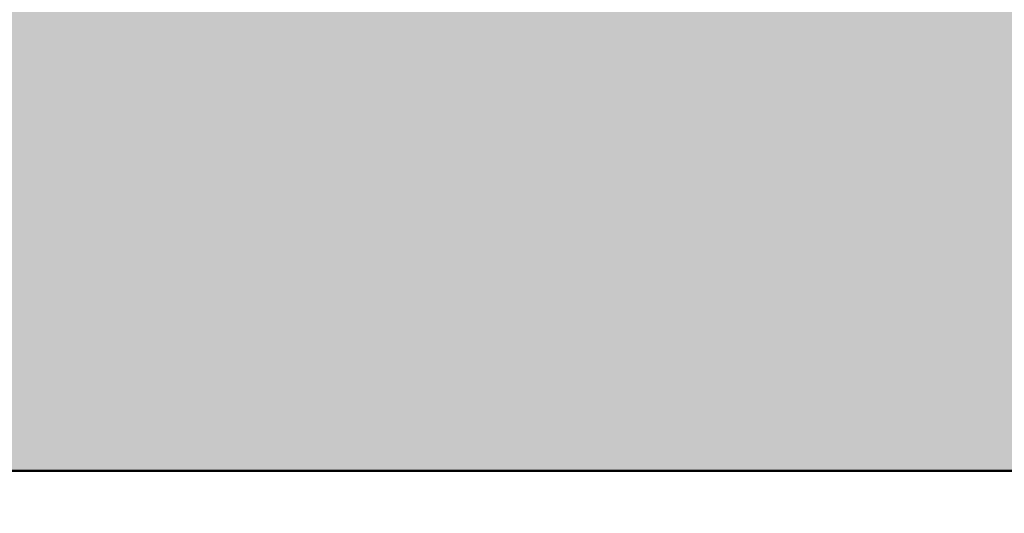
# Model space of a CAD drawing. Units: millimetres. Extents: x 0 to 2267, y 0 to 1823.
# Tile 26 of 256: x 1675 to 1760, y 1074 to 1117. Entities that reach past the tile are written whole.
import ezdxf

# ---------------------------------------------------------------- set-up
doc = ezdxf.new("R2010")
doc.units = ezdxf.units.MM
doc.header["$MEASUREMENT"] = 0
for name, color, linetype, lineweight in [('M-DIMS', 2, 'Continuous', 25), ('M-HATC', 252, 'Continuous', 18), ('M-OUTL', 7, 'Continuous', 50)]:
    doc.layers.add(name, color=color, linetype=linetype, lineweight=lineweight)
doc.styles.get("Standard").update_dxf_attribs({"font": 'arial.ttf'})
doc.dimstyles.get("Standard").update_dxf_attribs({"dimtxt": 7, "dimasz": 4, "dimexe": 0.18, "dimexo": 0.0625, "dimgap": 0.09, "dimtad": 0, "dimdec": 0, "dimzin": 0, "dimdsep": 46, "dimtxsty": 'Standard', "dimcen": 0.09, "dimadec": 0, "dimazin": 0, "dimtfac": 1, "dimtdec": 0, "dimtofl": 0, "dimtmove": 0, "dimatfit": 3, "dimfxl": 1, "dimtolj": 1, "dimtzin": 0, "dimarcsym": 0})

# ---------------------------------------------------------------- blocks, each defined once
blk = doc.blocks.new('*D1')
at = {"layer": 'Defpoints', "color": 0, "transparency": 16777216}
for p in [(1593.429, 1127.417), (1843.429, 1127.417), (1843.429, 955.628)]:
    blk.add_point(p, dxfattribs=at)
at = {"layer": 'M-DIMS', "color": 0, "lineweight": -2, "transparency": 16777216}
for p, q in [((1593.429, 1127.355), (1593.429, 955.448)), ((1843.429, 1127.355), (1843.429, 955.448)), ((1597.429, 955.628), (1710.558, 955.628)), ((1839.429, 955.628), (1726.3, 955.628))]:
    blk.add_line(p, q, dxfattribs=at)
at = {"layer": 'M-DIMS', "color": 0, "transparency": 16777216}
for points in [[(1597.429, 956.294), (1597.429, 954.961), (1593.429, 955.628)], [(1839.429, 956.294), (1839.429, 954.961), (1843.429, 955.628)]]:
    blk.add_solid(points, dxfattribs=at)
at = {"layer": 'M-DIMS', "color": 0, "transparency": 16777216, "insert": (1718.429, 955.628), "char_height": 7, "attachment_point": 5}
blk.add_mtext('\\A1;250', dxfattribs=at)
blk = doc.blocks.new('*D2')
at = {"layer": 'Defpoints', "color": 0, "transparency": 16777216}
for p in [(1505.929, 1077.417), (1930.929, 1077.417), (1930.929, 906.787)]:
    blk.add_point(p, dxfattribs=at)
at = {"layer": 'M-DIMS', "color": 0, "lineweight": -2, "transparency": 16777216}
for p, q in [((1505.929, 1077.355), (1505.929, 906.607)), ((1930.929, 1077.355), (1930.929, 906.607)), ((1509.929, 906.787), (1710.439, 906.787)), ((1926.929, 906.787), (1726.419, 906.787))]:
    blk.add_line(p, q, dxfattribs=at)
at = {"layer": 'M-DIMS', "color": 0, "transparency": 16777216}
for points in [[(1509.929, 907.453), (1509.929, 906.12), (1505.929, 906.787)], [(1926.929, 907.453), (1926.929, 906.12), (1930.929, 906.787)]]:
    blk.add_solid(points, dxfattribs=at)
at = {"layer": 'M-DIMS', "color": 0, "transparency": 16777216, "insert": (1718.429, 906.787), "char_height": 7, "attachment_point": 5}
blk.add_mtext('\\A1;425', dxfattribs=at)

msp = doc.modelspace()

# ---------------------------------------------------------------- hatches: boundary and pattern name
at = {"layer": 'M-HATC'}
h = msp.add_hatch(color=256, dxfattribs=at)
h.dxf.hatch_style = 1
h.paths.add_polyline_path([(2065.771, 1618.062, 0.236068), (2055.771, 1638.062), (1381.087, 1638.062, 0.236068), (1371.087, 1618.062), (1371.087, 1603.062), (2055.771, 1603.062), (2065.771, 1603.062)])
h.paths.add_polyline_path([(2062.772, 1550.296), (2062.772, 1560.296), (1374.086, 1560.296), (1374.086, 1550.296), (1374.086, 1540.296), (1384.086, 1540.296), (1389.086, 1540.296), (2062.772, 1540.296)])
h.paths.add_polyline_path([(1930.929, 1282.766), (1505.929, 1282.766), (1587.628, 1235.597, 0.131652), (1600.128, 1232.247), (1836.73, 1232.247, 0.131652), (1849.23, 1235.597)])
h.paths.add_polyline_path([(1930.929, 1117.417), (1905.929, 1117.417), (1505.929, 1117.417), (1505.929, 1077.417), (1930.929, 1077.417)])

# ---------------------------------------------------------------- linework, layer by layer
at = {"layer": 'M-OUTL'}
msp.add_line((1505.929, 1077.417), (1930.929, 1077.417), dxfattribs=at)

# ---------------------------------------------------------------- dimensions: what is measured, and where the dimension line sits
at = {"layer": 'M-DIMS'}
for base, p1, p2, picture, middle in [((1843.429, 955.628), (1593.429, 1127.417), (1843.429, 1127.417), '*D1', (1718.429, 955.628)), ((1930.929, 906.787), (1505.929, 1077.417), (1930.929, 1077.417), '*D2', (1718.429, 906.787))]:
    dim = msp.add_linear_dim(base=base, p1=p1, p2=p2, dimstyle='Standard', override={"dimclrd": 0, "dimclre": 0, "dimclrt": 0}, dxfattribs=at)
    dim.commit()
    dim.dimension.update_dxf_attribs({"geometry": picture, "text_midpoint": middle})

doc.saveas('drawing.dxf')
